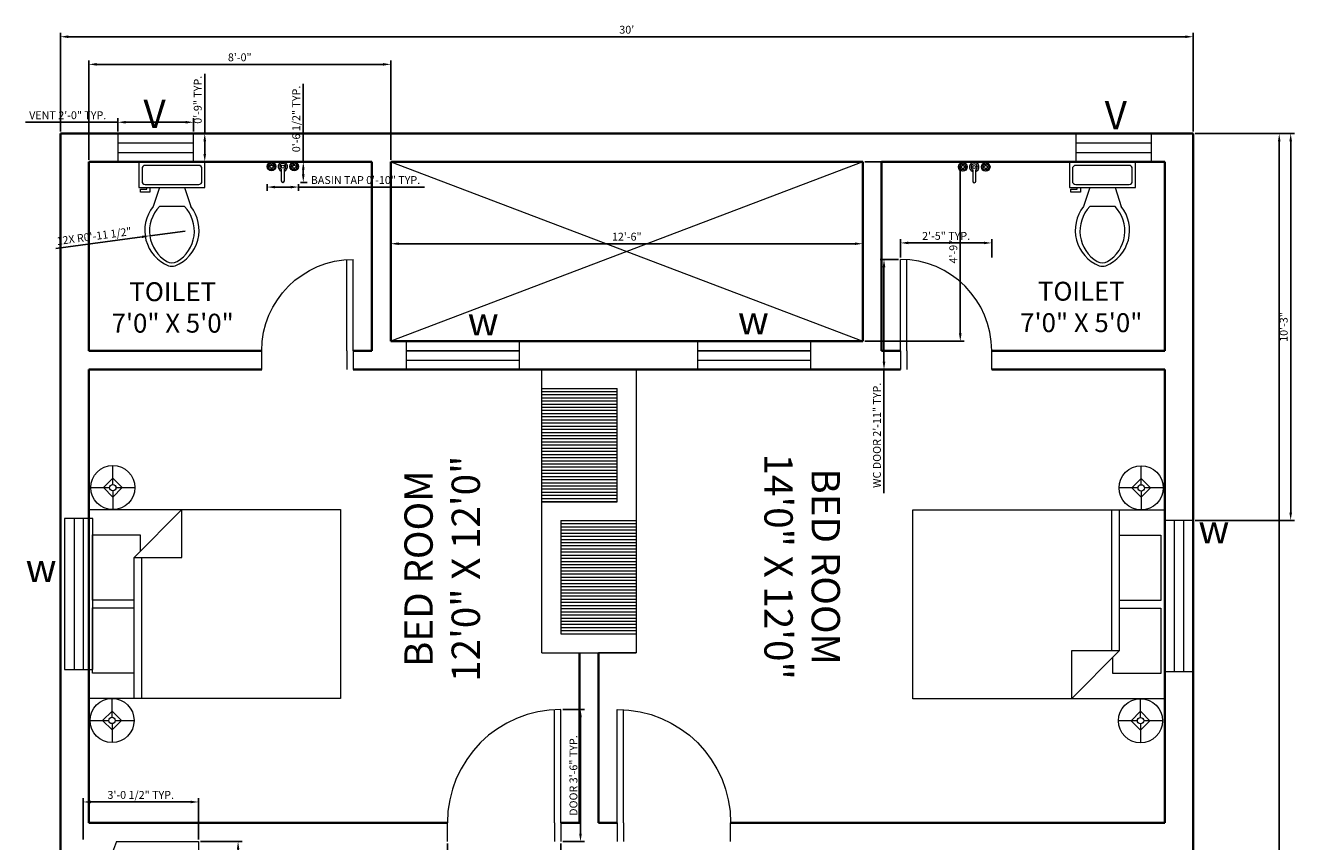
# Model space of a CAD drawing. Units: inches. Extents: x 2009 to 2890, y 2827 to 3504.
# Tile 6 of 6: x 2486 to 2890, y 3214 to 3473. Entities that reach past the tile are written whole.
import ezdxf

# ---------------------------------------------------------------- set-up
doc = ezdxf.new("R2010")
doc.units = ezdxf.units.IN
for name, color, linetype, lineweight in [('A-ANNO-DIMS', 2, 'Continuous', 18), ('A-ANNO-TEXT', 3, 'Continuous', 18), ('A-AREA-IDEN', 7, 'Continuous', 25), ('A-DOOR', 3, 'Continuous', 18), ('A-FLOR-CASE', 32, 'Continuous', 20), ('A-FLOR-FIXT', 9, 'Continuous', 18), ('A-FLOR-OPEN', 8, 'Continuous', 13), ('A-FLOR-PATT', 252, 'Continuous', 13), ('A-FURN', 8, 'Continuous', 18), ('A-GLAZ', 4, 'Continuous', 18), ('A-WALL', 7, 'Continuous', 35)]:
    doc.layers.add(name, color=color, linetype=linetype, lineweight=lineweight)
doc.styles.get("Standard").update_dxf_attribs({"font": 'arial.ttf'})
doc.dimstyles.new('ISO-25', dxfattribs={"dimtxt": 2.5, "dimasz": 2.5, "dimexe": 1.25, "dimexo": 0.625, "dimtad": 1, "dimdec": 0, "dimlunit": 3, "dimtxsty": 'Standard', "dimcen": 2.5, "dimadec": 0, "dimazin": 0, "dimtfac": 1, "dimtdec": 0, "dimtmove": 0, "dimatfit": 3, "dimfxl": 1, "dimarcsym": 0})

# ---------------------------------------------------------------- blocks, each defined once
blk = doc.blocks.new('*D13')
at = {"layer": 'A-ANNO-DIMS', "color": 0, "lineweight": -2, "transparency": 16777216}
for p, q in [((2497.61, 3439.57), (2497.61, 3470.97)), ((2500.11, 3469.72), (2855.11, 3469.72)), ((2857.61, 3439.57), (2857.61, 3470.97))]:
    blk.add_line(p, q, dxfattribs=at)
at = {"layer": 'A-ANNO-DIMS', "color": 0, "transparency": 16777216}
for points in [[(2500.11, 3470.14), (2500.11, 3469.3), (2497.61, 3469.72)], [(2855.11, 3470.14), (2855.11, 3469.3), (2857.61, 3469.72)]]:
    blk.add_solid(points, dxfattribs=at)
at = {"layer": 'Defpoints', "color": 0, "transparency": 16777216}
for p in [(2857.61, 3469.72), (2497.61, 3438.94), (2857.61, 3438.94)]:
    blk.add_point(p, dxfattribs=at)
at = {"layer": 'A-ANNO-DIMS', "color": 0, "transparency": 16777216, "insert": (2677.61, 3471.62), "char_height": 2.5, "attachment_point": 5}
blk.add_mtext("30'", dxfattribs=at)
blk = doc.blocks.new('*D14')
at = {"layer": 'A-ANNO-DIMS', "color": 0, "lineweight": -2, "transparency": 16777216}
for p, q in [((2858.24, 3438.94), (2886.22, 3438.94)), ((2884.97, 3436.44), (2884.97, 2901.44)), ((2870.41, 2898.94), (2886.22, 2898.94))]:
    blk.add_line(p, q, dxfattribs=at)
at = {"layer": 'A-ANNO-DIMS', "color": 0, "transparency": 16777216}
for points in [[(2884.55, 3436.44), (2885.39, 3436.44), (2884.97, 3438.94)], [(2884.55, 2901.44), (2885.39, 2901.44), (2884.97, 2898.94)]]:
    blk.add_solid(points, dxfattribs=at)
at = {"layer": 'Defpoints', "color": 0, "transparency": 16777216}
for p in [(2857.61, 3438.94), (2869.79, 2898.94), (2884.97, 2898.94)]:
    blk.add_point(p, dxfattribs=at)
at = {"layer": 'A-ANNO-DIMS', "color": 0, "transparency": 16777216, "insert": (2883.07, 3168.94), "char_height": 2.5, "attachment_point": 5, "rotation": 90}
blk.add_mtext("45'", dxfattribs=at)
blk = doc.blocks.new('Toilet - top')
for p, q in [((9.5, -6), (9.5, -2)), ((-8, -8.5), (-8, -8)), ((-7, -8), (-7, -9.5)), ((-4, -8), (-6, -14)), ((4, -8), (6, -14)), ((-10, -8.5), (-8, -8.5)), ((-10, -9.5), (-10, -8.5)), ((-7, -9.5), (-10, -9.5)), ((4, -14), (-4, -14))]:
    blk.add_line(p, q)
blk.add_lwpolyline([(10.5, -8), (10.5, 0), (-10.5, 0), (-10.5, -8)], close=True)
for points in [[(-9.5, -2), (-9.5, -6)], [(8.5, -1), (-8.5, -1)], [(-8.5, -7), (8.5, -7)]]:
    blk.add_lwpolyline(points)
for centre, radius, start, end in [((-8.62, -1.88), 0.884, 81.8699, 188.1301), ((8.62, -1.88), 0.884, 351.8699, 98.1301), ((-8.62, -6.12), 0.884, 171.8699, 278.1301), ((8.62, -6.12), 0.884, 261.8699, 8.1301), ((3.52, -21.58), 12.17, 141.4691, 247.9714), ((4.2, -21.82), 11.33, 136.3677, 238.9468), ((-3.52, -21.58), 12.17, 292.0284, 38.5307), ((-4.2, -21.82), 11.33, 301.053, 43.6321), ((0, -27.88), 4, 245.7318, 294.2682), ((0, -29), 4, 254.8605, 285.1395)]:
    blk.add_arc(centre, radius, start, end)
blk = doc.blocks.new('Sofa - Roundback 7 ft.')
for p, q in [((-12.00002, -32.4421), (-12.00003, -6.5971)), ((11.99997, -32.4421), (11.99998, -6.5971)), ((-36.000027, -34), (-36.000027, -11.4696)), ((35.99998, -34), (35.99998, -11.4696)), ((-35.999844, -13.3819), (35.9998, -13.3819)), ((-36.000027, -32.4421), (35.99998, -32.4421))]:
    blk.add_line(p, q)
for points in [[(-36.000027, -34), (-42.000027, -34), (-42.000027, -8)], [(41.99998, -8), (41.99998, -34), (35.99998, -34)]]:
    blk.add_lwpolyline(points)
for centre, radius, start, end in [((0, -114.25), 114.25, 68.43141, 111.5686), ((-0.00001, -127.1968), 121.1968, 72.72033, 107.2797)]:
    blk.add_arc(centre, radius, start, end)
blk = doc.blocks.new('Bed - Queen')
for p, q in [((0, -80.00003), (0, 0)), ((0, 0), (59.99999, 0)), ((59.99999, 0), (59.99999, -80.00003)), ((7.99999, -1.2), (28.79998, -1.2)), ((7.99999, -14.4), (7.99999, -1.2)), ((28.79998, -1.2), (28.79998, -14.4)), ((31.19999, -1.2), (51.99999, -1.2)), ((31.19999, -14.4), (31.19999, -1.2)), ((51.99999, -1.2), (51.99999, -16.4)), ((0, -14.4), (44.8, -14.4)), ((59.99999, -29.6), (44.8, -14.4)), ((44.8, -14.4), (44.8, -29.6)), ((44.8, -16.8), (0, -16.8)), ((51.99999, -16.4), (46.79936, -16.4)), ((44.8, -29.6), (59.99999, -29.6)), ((59.99999, -80.00003), (0, -80.00003))]:
    blk.add_line(p, q)
blk = doc.blocks.new('Lamp - Table')
for p, q in [((0, 7), (0, 1)), ((-1, 0), (-7, 0)), ((0, 3), (-3, 0)), ((-3, 0), (0, -3)), ((3, 0), (0, 3)), ((0, -3), (3, 0)), ((1, 0), (7, 0)), ((0, -1), (0, -7))]:
    blk.add_line(p, q)
for radius in [7, 1]:
    blk.add_circle((0, 0), radius)
blk = doc.blocks.new('Faucet - Bathroom top')
for p, q in [((-4.107, 0.125), (-4.375, 0.125)), ((-3.75, 0.4788), (-3.75, 0.75)), ((-3.5, 0.482), (-3.5, 0.75)), ((-3.1461, 0.125), (-2.875, 0.125)), ((3.143, 0.125), (2.875, 0.125)), ((3.5, 0.4788), (3.5, 0.75)), ((3.75, 0.482), (3.75, 0.75)), ((4.1039, 0.125), (4.375, 0.125)), ((-4.1039, -0.125), (-4.375, -0.125)), ((-3.75, -0.4821), (-3.75, -0.75)), ((-3.5, -0.4789), (-3.5, -0.75)), ((-3.143, -0.125), (-2.875, -0.125)), ((-0.5, -0.8639), (-0.5, -4.5)), ((0.5, -4.5), (0.5, -0.8631)), ((3.1461, -0.125), (2.875, -0.125)), ((3.5, -0.4821), (3.5, -0.75)), ((3.75, -0.4789), (3.75, -0.75)), ((4.107, -0.125), (4.375, -0.125))]:
    blk.add_line(p, q)
for centre, radius in [((-3.625, 0), 1.375), ((-4.625, 0), 0.2795), ((-3.625, 0), 0.5), ((-3.625, 1), 0.2795), ((-2.625, 0), 0.2795), ((0, 0), 0.5), ((3.625, 0), 1.375), ((2.625, 0), 0.2795), ((3.625, 0), 0.5), ((3.625, 1), 0.2795), ((4.625, 0), 0.2795), ((-3.625, -1), 0.2795), ((3.625, -1), 0.2795)]:
    blk.add_circle(centre, radius)
for centre, radius, start, end in [((-3.625, 0), 1, 105.2407, 164.2093), ((-3.625, 0), 1, 16.44125, 74.07887), ((0, 0), 1.5, 289.6514, 250.3603), ((0, 0), 1, 300.3431, 239.7554), ((3.625, 0), 1, 106.12, 164.0884), ((3.625, 0), 1, 16.23422, 73.90469), ((-3.625, 0), 1, 196.2342, 253.9047), ((-3.625, 0), 1, 286.12, 344.0884), ((3.625, 0), 1, 196.4413, 254.0789), ((3.625, 0), 1, 285.2407, 344.2093), ((0, -4.5), 0.5, 180, 0)]:
    blk.add_arc(centre, radius, start, end)
blk = doc.blocks.new('WIN-48IN')
for p, q in [((0, 48), (0, 0)), ((9, 48), (0, 48)), ((3, 48), (3, 0)), ((6, 0), (6, 48)), ((9, 0), (9, 48)), ((0, 0), (9, 0))]:
    blk.add_line(p, q)
blk = doc.blocks.new('WIN-36IN')
for p, q in [((0, 36), (0, 0)), ((9, 36), (0, 36)), ((3, 36), (3, 0)), ((6, 0), (6, 36)), ((9, 0), (9, 36)), ((0, 0), (9, 0))]:
    blk.add_line(p, q)
blk = doc.blocks.new('VENT-24IN')
for p, q in [((0, 24), (0, 0)), ((9, 24), (0, 24)), ((3, 24), (3, 0)), ((6, 0), (6, 24)), ((9, 0), (9, 24)), ((0, 0), (9, 0))]:
    blk.add_line(p, q)
blk = doc.blocks.new('DOOR-29IN')
for p, q in [((0, 35), (0, 29)), ((27, 29), (27, 35)), ((29, 29), (29, 35)), ((27, 29), (27, 0)), ((29, 29), (29, 0))]:
    blk.add_line(p, q)
blk.add_arc((29, 29), 29, 180, 270)
blk = doc.blocks.new('DOOR-36IN')
for p, q in [((34, 6), (34, 42)), ((36, 6), (36, 42)), ((0, 0), (0, 6)), ((34, 6), (34, 0)), ((36, 6), (36, 0))]:
    blk.add_line(p, q)
blk.add_arc((36, 6), 36, 90, 180)
blk = doc.blocks.new('*D35')
at = {"layer": 'A-ANNO-DIMS', "color": 0, "lineweight": -2, "transparency": 16777216}
for p, q in [((2515.89, 3442.54), (2486.48, 3442.54)), ((2515.89, 3439.57), (2515.89, 3443.79)), ((2537.39, 3442.54), (2518.39, 3442.54)), ((2539.89, 3439.57), (2539.89, 3443.79))]:
    blk.add_line(p, q, dxfattribs=at)
at = {"layer": 'A-ANNO-DIMS', "color": 0, "transparency": 16777216}
for points in [[(2518.39, 3442.96), (2518.39, 3442.13), (2515.89, 3442.54)], [(2537.39, 3442.96), (2537.39, 3442.13), (2539.89, 3442.54)]]:
    blk.add_solid(points, dxfattribs=at)
at = {"layer": 'Defpoints', "color": 0, "transparency": 16777216}
for p in [(2515.89, 3442.54), (2515.89, 3438.94), (2539.89, 3438.94)]:
    blk.add_point(p, dxfattribs=at)
at = {"layer": 'A-ANNO-DIMS', "color": 0, "transparency": 16777216, "insert": (2499.94, 3444.45), "char_height": 2.5, "attachment_point": 5}
blk.add_mtext('VENT 2\'-0" TYP.', dxfattribs=at)
blk = doc.blocks.new('*D36')
at = {"layer": 'A-ANNO-DIMS', "color": 0, "lineweight": -2, "transparency": 16777216}
for p, q in [((2543.49, 3438.94), (2543.49, 3457.93)), ((2540.51, 3438.94), (2544.74, 3438.94)), ((2543.49, 3432.44), (2543.49, 3436.44)), ((2540.51, 3429.94), (2544.74, 3429.94))]:
    blk.add_line(p, q, dxfattribs=at)
at = {"layer": 'A-ANNO-DIMS', "color": 0, "transparency": 16777216}
for points in [[(2543.07, 3436.44), (2543.9, 3436.44), (2543.49, 3438.94)], [(2543.07, 3432.44), (2543.9, 3432.44), (2543.49, 3429.94)]]:
    blk.add_solid(points, dxfattribs=at)
at = {"layer": 'Defpoints', "color": 0, "transparency": 16777216}
for p in [(2539.89, 3438.94), (2543.49, 3438.94), (2539.89, 3429.94)]:
    blk.add_point(p, dxfattribs=at)
at = {"layer": 'A-ANNO-DIMS', "color": 0, "transparency": 16777216, "insert": (2541.59, 3449.69), "char_height": 2.5, "attachment_point": 5, "rotation": 90}
blk.add_mtext('0\'-9" TYP.', dxfattribs=at)
blk = doc.blocks.new('*D37')
at = {"layer": 'A-ANNO-DIMS', "color": 0, "lineweight": -2, "transparency": 16777216}
for p, q in [((2657.24, 3255.94), (2664.16, 3255.94)), ((2662.91, 3216.44), (2662.91, 3253.44)), ((2657.24, 3213.94), (2664.16, 3213.94))]:
    blk.add_line(p, q, dxfattribs=at)
at = {"layer": 'A-ANNO-DIMS', "color": 0, "transparency": 16777216}
for points in [[(2662.49, 3253.44), (2663.33, 3253.44), (2662.91, 3255.94)], [(2662.49, 3216.44), (2663.33, 3216.44), (2662.91, 3213.94)]]:
    blk.add_solid(points, dxfattribs=at)
at = {"layer": 'Defpoints', "color": 0, "transparency": 16777216}
for p in [(2656.61, 3255.94), (2662.91, 3255.94), (2656.61, 3213.94)]:
    blk.add_point(p, dxfattribs=at)
at = {"layer": 'A-ANNO-DIMS', "color": 0, "transparency": 16777216, "insert": (2660.99, 3234.94), "char_height": 2.5, "attachment_point": 5, "rotation": 90}
blk.add_mtext('DOOR 3\'-6" TYP.', dxfattribs=at)
blk = doc.blocks.new('*D38')
at = {"layer": 'A-ANNO-DIMS', "color": 0, "lineweight": -2, "transparency": 16777216}
for p, q in [((2620.61, 3213.32), (2620.61, 3206.39)), ((2656.61, 3213.32), (2656.61, 3206.39)), ((2623.11, 3207.64), (2654.11, 3207.64))]:
    blk.add_line(p, q, dxfattribs=at)
at = {"layer": 'A-ANNO-DIMS', "color": 0, "transparency": 16777216}
for points in [[(2623.11, 3208.06), (2623.11, 3207.23), (2620.61, 3207.64)], [(2654.11, 3208.06), (2654.11, 3207.23), (2656.61, 3207.64)]]:
    blk.add_solid(points, dxfattribs=at)
at = {"layer": 'Defpoints', "color": 0, "transparency": 16777216}
for p in [(2620.61, 3213.94), (2656.61, 3213.94), (2656.61, 3207.64)]:
    blk.add_point(p, dxfattribs=at)
at = {"layer": 'A-ANNO-DIMS', "color": 0, "transparency": 16777216, "insert": (2638.61, 3209.55), "char_height": 2.5, "attachment_point": 5}
blk.add_mtext('3\'-0" TYP.', dxfattribs=at)
blk = doc.blocks.new('*D39')
at = {"layer": 'A-ANNO-DIMS', "color": 0, "lineweight": -2, "transparency": 16777216}
for p, q in [((2763.99, 3398.94), (2758.11, 3398.94)), ((2759.36, 3396.44), (2759.36, 3366.44)), ((2763.99, 3363.94), (2758.11, 3363.94)), ((2759.36, 3363.94), (2759.36, 3324.67))]:
    blk.add_line(p, q, dxfattribs=at)
at = {"layer": 'A-ANNO-DIMS', "color": 0, "transparency": 16777216}
for points in [[(2758.94, 3396.44), (2759.78, 3396.44), (2759.36, 3398.94)], [(2758.94, 3366.44), (2759.78, 3366.44), (2759.36, 3363.94)]]:
    blk.add_solid(points, dxfattribs=at)
at = {"layer": 'Defpoints', "color": 0, "transparency": 16777216}
for p in [(2764.61, 3398.94), (2759.36, 3363.94), (2764.61, 3363.94)]:
    blk.add_point(p, dxfattribs=at)
at = {"layer": 'A-ANNO-DIMS', "color": 0, "transparency": 16777216, "insert": (2757.44, 3343.06), "char_height": 2.5, "attachment_point": 5, "rotation": 90}
blk.add_mtext('WC DOOR 2\'-11" TYP.', dxfattribs=at)
blk = doc.blocks.new('*D40')
at = {"layer": 'A-ANNO-DIMS', "color": 0, "lineweight": -2, "transparency": 16777216}
for p, q in [((2764.61, 3399.57), (2764.61, 3405.44)), ((2793.61, 3399.57), (2793.61, 3405.44)), ((2791.11, 3404.19), (2767.11, 3404.19))]:
    blk.add_line(p, q, dxfattribs=at)
at = {"layer": 'A-ANNO-DIMS', "color": 0, "transparency": 16777216}
for points in [[(2767.11, 3404.61), (2767.11, 3403.78), (2764.61, 3404.19)], [(2791.11, 3404.61), (2791.11, 3403.78), (2793.61, 3404.19)]]:
    blk.add_solid(points, dxfattribs=at)
at = {"layer": 'Defpoints', "color": 0, "transparency": 16777216}
for p in [(2764.61, 3404.19), (2764.61, 3398.94), (2793.61, 3398.94)]:
    blk.add_point(p, dxfattribs=at)
at = {"layer": 'A-ANNO-DIMS', "color": 0, "transparency": 16777216, "insert": (2779.11, 3406.1), "char_height": 2.5, "attachment_point": 5}
blk.add_mtext('2\'-5" TYP.', dxfattribs=at)
blk = doc.blocks.new('*D49')
at = {"layer": 'A-ANNO-DIMS', "color": 0, "lineweight": -2, "transparency": 16777216}
for p, q in [((2563.31, 3422.82), (2563.31, 3420.7)), ((2565.81, 3421.95), (2570.81, 3421.95)), ((2573.31, 3422.82), (2573.31, 3420.7)), ((2573.31, 3421.95), (2613.34, 3421.95))]:
    blk.add_line(p, q, dxfattribs=at)
at = {"layer": 'A-ANNO-DIMS', "color": 0, "transparency": 16777216}
for points in [[(2565.81, 3422.36), (2565.81, 3421.53), (2563.31, 3421.95)], [(2570.81, 3422.36), (2570.81, 3421.53), (2573.31, 3421.95)]]:
    blk.add_solid(points, dxfattribs=at)
at = {"layer": 'Defpoints', "color": 0, "transparency": 16777216}
for p in [(2563.31, 3423.45), (2573.31, 3423.45), (2573.31, 3421.95)]:
    blk.add_point(p, dxfattribs=at)
at = {"layer": 'A-ANNO-DIMS', "color": 0, "transparency": 16777216, "insert": (2594.57, 3423.86), "char_height": 2.5, "attachment_point": 5}
blk.add_mtext('BASIN TAP 0\'-10" TYP.', dxfattribs=at)
blk = doc.blocks.new('*D50')
at = {"layer": 'A-ANNO-DIMS', "color": 0, "lineweight": -2, "transparency": 16777216}
for p, q in [((2574.81, 3429.95), (2574.81, 3454.76)), ((2573.93, 3429.95), (2576.06, 3429.95)), ((2574.81, 3425.95), (2574.81, 3427.45)), ((2573.93, 3423.45), (2576.06, 3423.45))]:
    blk.add_line(p, q, dxfattribs=at)
at = {"layer": 'A-ANNO-DIMS', "color": 0, "transparency": 16777216}
for points in [[(2574.39, 3427.45), (2575.22, 3427.45), (2574.81, 3429.95)], [(2574.39, 3425.95), (2575.22, 3425.95), (2574.81, 3423.45)]]:
    blk.add_solid(points, dxfattribs=at)
at = {"layer": 'Defpoints', "color": 0, "transparency": 16777216}
for p in [(2573.31, 3429.95), (2574.81, 3429.95), (2573.31, 3423.45)]:
    blk.add_point(p, dxfattribs=at)
at = {"layer": 'A-ANNO-DIMS', "color": 0, "transparency": 16777216, "insert": (2572.89, 3443.6), "char_height": 2.5, "attachment_point": 5, "rotation": 90}
blk.add_mtext('0\'-6 1/2" TYP.', dxfattribs=at)
blk = doc.blocks.new('*D51')
at = {"layer": 'A-ANNO-DIMS', "color": 0, "lineweight": -2, "transparency": 16777216}
for p, q in [((2542.11, 3213.94), (2555.33, 3213.94)), ((2554.08, 3132.44), (2554.08, 3211.44)), ((2542.11, 3129.94), (2555.33, 3129.94))]:
    blk.add_line(p, q, dxfattribs=at)
at = {"layer": 'A-ANNO-DIMS', "color": 0, "transparency": 16777216}
for points in [[(2553.67, 3211.44), (2554.5, 3211.44), (2554.08, 3213.94)], [(2553.67, 3132.44), (2554.5, 3132.44), (2554.08, 3129.94)]]:
    blk.add_solid(points, dxfattribs=at)
at = {"layer": 'Defpoints', "color": 0, "transparency": 16777216}
for p in [(2541.48, 3213.94), (2554.08, 3213.94), (2541.48, 3129.94)]:
    blk.add_point(p, dxfattribs=at)
at = {"layer": 'A-ANNO-DIMS', "color": 0, "transparency": 16777216, "insert": (2552.16, 3171.94), "char_height": 2.5, "attachment_point": 5, "rotation": 90}
blk.add_mtext('SOFA 7\'-0" TYP.', dxfattribs=at)
blk = doc.blocks.new('*D52')
at = {"layer": 'A-ANNO-DIMS', "color": 0, "lineweight": -2, "transparency": 16777216}
for p, q in [((2504.82, 3214.57), (2504.82, 3227.79)), ((2541.48, 3214.57), (2541.48, 3227.79)), ((2538.98, 3226.54), (2507.32, 3226.54))]:
    blk.add_line(p, q, dxfattribs=at)
at = {"layer": 'A-ANNO-DIMS', "color": 0, "transparency": 16777216}
for points in [[(2507.32, 3226.96), (2507.32, 3226.13), (2504.82, 3226.54)], [(2538.98, 3226.96), (2538.98, 3226.13), (2541.48, 3226.54)]]:
    blk.add_solid(points, dxfattribs=at)
at = {"layer": 'Defpoints', "color": 0, "transparency": 16777216}
for p in [(2504.82, 3226.54), (2504.82, 3213.94), (2541.48, 3213.94)]:
    blk.add_point(p, dxfattribs=at)
at = {"layer": 'A-ANNO-DIMS', "color": 0, "transparency": 16777216, "insert": (2523.15, 3228.46), "char_height": 2.5, "attachment_point": 5}
blk.add_mtext('3\'-0 1/2" TYP.', dxfattribs=at)
blk = doc.blocks.new('*D70')
at = {"layer": 'A-ANNO-DIMS', "color": 0, "lineweight": -2, "transparency": 16777216}
for p, q in [((2602.61, 3373.57), (2602.61, 3405.19)), ((2752.61, 3373.57), (2752.61, 3405.19)), ((2605.11, 3403.94), (2750.11, 3403.94))]:
    blk.add_line(p, q, dxfattribs=at)
at = {"layer": 'A-ANNO-DIMS', "color": 0, "transparency": 16777216}
for points in [[(2605.11, 3404.36), (2605.11, 3403.53), (2602.61, 3403.94)], [(2750.11, 3404.36), (2750.11, 3403.53), (2752.61, 3403.94)]]:
    blk.add_solid(points, dxfattribs=at)
at = {"layer": 'Defpoints', "color": 0, "transparency": 16777216}
for p in [(2752.61, 3403.94), (2602.61, 3372.94), (2752.61, 3372.94)]:
    blk.add_point(p, dxfattribs=at)
at = {"layer": 'A-ANNO-DIMS', "color": 0, "transparency": 16777216, "insert": (2677.61, 3405.85), "char_height": 2.5, "attachment_point": 5}
blk.add_mtext('12\'-6"', dxfattribs=at)
blk = doc.blocks.new('*D71')
at = {"layer": 'A-ANNO-DIMS', "color": 0, "lineweight": -2, "transparency": 16777216}
for p, q in [((2753.24, 3429.94), (2784.86, 3429.94)), ((2783.61, 3427.44), (2783.61, 3375.44)), ((2753.24, 3372.94), (2784.86, 3372.94))]:
    blk.add_line(p, q, dxfattribs=at)
at = {"layer": 'A-ANNO-DIMS', "color": 0, "transparency": 16777216}
for points in [[(2783.19, 3427.44), (2784.03, 3427.44), (2783.61, 3429.94)], [(2783.19, 3375.44), (2784.03, 3375.44), (2783.61, 3372.94)]]:
    blk.add_solid(points, dxfattribs=at)
at = {"layer": 'Defpoints', "color": 0, "transparency": 16777216}
for p in [(2752.61, 3429.94), (2752.61, 3372.94), (2783.61, 3372.94)]:
    blk.add_point(p, dxfattribs=at)
at = {"layer": 'A-ANNO-DIMS', "color": 0, "transparency": 16777216, "insert": (2781.71, 3401.44), "char_height": 2.5, "attachment_point": 5, "rotation": 90}
blk.add_mtext('4\'-9"', dxfattribs=at)
blk = doc.blocks.new('*D78')
at = {"layer": 'A-ANNO-DIMS', "color": 0, "lineweight": -2, "transparency": 16777216}
for p, q in [((2506.61, 3430.57), (2506.61, 3462.19)), ((2602.61, 3430.57), (2602.61, 3462.19)), ((2509.11, 3460.94), (2600.11, 3460.94))]:
    blk.add_line(p, q, dxfattribs=at)
at = {"layer": 'A-ANNO-DIMS', "color": 0, "transparency": 16777216}
for points in [[(2509.11, 3461.36), (2509.11, 3460.53), (2506.61, 3460.94)], [(2600.11, 3461.36), (2600.11, 3460.53), (2602.61, 3460.94)]]:
    blk.add_solid(points, dxfattribs=at)
at = {"layer": 'Defpoints', "color": 0, "transparency": 16777216}
for p in [(2602.61, 3460.94), (2506.61, 3429.94), (2602.61, 3429.94)]:
    blk.add_point(p, dxfattribs=at)
at = {"layer": 'A-ANNO-DIMS', "color": 0, "transparency": 16777216, "insert": (2554.61, 3462.85), "char_height": 2.5, "attachment_point": 5}
blk.add_mtext('8\'-0"', dxfattribs=at)
blk = doc.blocks.new('*D82')
at = {"layer": 'A-ANNO-DIMS', "color": 0, "lineweight": -2, "transparency": 16777216}
for p, q in [((2858.24, 3438.94), (2889.86, 3438.94)), ((2888.61, 3436.44), (2888.61, 3318.53)), ((2858.24, 3316.03), (2889.86, 3316.03))]:
    blk.add_line(p, q, dxfattribs=at)
at = {"layer": 'A-ANNO-DIMS', "color": 0, "transparency": 16777216}
for points in [[(2888.19, 3436.44), (2889.03, 3436.44), (2888.61, 3438.94)], [(2888.19, 3318.53), (2889.03, 3318.53), (2888.61, 3316.03)]]:
    blk.add_solid(points, dxfattribs=at)
at = {"layer": 'Defpoints', "color": 0, "transparency": 16777216}
for p in [(2857.61, 3438.94), (2857.61, 3316.03), (2888.61, 3316.03)]:
    blk.add_point(p, dxfattribs=at)
at = {"layer": 'A-ANNO-DIMS', "color": 0, "transparency": 16777216, "insert": (2886.71, 3377.49), "char_height": 2.5, "attachment_point": 5, "rotation": 90}
blk.add_mtext('10\'-3"', dxfattribs=at)
blk = doc.blocks.new('*D92')
at = {"layer": 'A-ANNO-DIMS', "color": 0, "lineweight": -2, "transparency": 16777216}
for p, q in [((2496.16, 3402.45), (2523.55, 3406.13)), ((2537.26, 3407.97), (2526.03, 3406.47))]:
    blk.add_line(p, q, dxfattribs=at)
at = {"layer": 'A-ANNO-DIMS', "color": 0, "transparency": 16777216}
blk.add_solid([(2523.49, 3406.54), (2523.6, 3405.72), (2526.03, 3406.47)], dxfattribs=at)
at = {"layer": 'Defpoints', "color": 0, "transparency": 16777216}
for p in [(2526.03, 3406.47), (2537.26, 3407.97)]:
    blk.add_point(p, dxfattribs=at)
at = {"layer": 'A-ANNO-DIMS', "color": 0, "transparency": 16777216, "insert": (2508.36, 3406.02), "char_height": 2.5, "attachment_point": 5, "rotation": 7.6592}
blk.add_mtext('12X R0\'-11 1/2"', dxfattribs=at)

msp = doc.modelspace()

# ---------------------------------------------------------------- hatches: boundary and pattern name
at = {"layer": 'A-FLOR-PATT'}
h = msp.add_hatch(dxfattribs=at)
h.set_pattern_fill('ANSI31', color=256, scale=0.3149606, angle=-45, style=0)
h.paths.add_polyline_path([(2650.61, 3321.94), (2674.61, 3321.94), (2674.61, 3357.94), (2650.61, 3357.94)])
h = msp.add_hatch(dxfattribs=at)
h.set_pattern_fill('ANSI31', color=256, scale=0.3149606, angle=-45, style=0)
h.paths.add_polyline_path([(2656.61, 3279.94), (2680.61, 3279.94), (2680.61, 3315.94), (2656.61, 3315.94)])

# ---------------------------------------------------------------- linework, layer by layer
at = {"layer": 'A-FLOR-CASE'}
for p, q in [((2650.61, 3273.94), (2650.61, 3363.94)), ((2680.61, 3363.94), (2680.61, 3273.94)), ((2650.61, 3357.94), (2674.61, 3357.94)), ((2674.61, 3321.94), (2674.61, 3357.94)), ((2650.61, 3321.94), (2674.61, 3321.94)), ((2656.61, 3315.94), (2680.61, 3315.94)), ((2656.61, 3315.94), (2656.61, 3279.94)), ((2656.61, 3279.94), (2680.61, 3279.94)), ((2650.61, 3273.94), (2680.61, 3273.94)), ((2650.61, 3273.94), (2662.61, 3273.94)), ((2680.61, 3273.94), (2668.61, 3273.94))]:
    msp.add_line(p, q, dxfattribs=at)
at = {"layer": 'A-FLOR-OPEN'}
for p, q in [((2602.61, 3429.94), (2752.61, 3372.94)), ((2752.61, 3429.94), (2602.61, 3372.94))]:
    msp.add_line(p, q, dxfattribs=at)
at = {"layer": 'A-GLAZ'}
for p, q in [((2607.51, 3369.94), (2643.51, 3369.94)), ((2700.1, 3369.94), (2736.1, 3369.94))]:
    msp.add_line(p, q, dxfattribs=at)
at = {"layer": 'A-WALL'}
for p, q in [((2497.61, 3438.94), (2857.61, 3438.94)), ((2497.61, 2898.94), (2497.61, 3438.94)), ((2857.61, 3438.94), (2857.61, 2898.94)), ((2506.61, 3429.94), (2596.61, 3429.94)), ((2506.61, 3369.94), (2506.61, 3429.94)), ((2596.61, 3369.94), (2596.61, 3429.94)), ((2602.61, 3372.94), (2602.61, 3429.94)), ((2602.61, 3429.94), (2752.61, 3429.94)), ((2752.61, 3429.94), (2752.61, 3372.94)), ((2752.61, 3372.94), (2752.61, 3429.94)), ((2752.61, 3372.94), (2752.61, 3429.94)), ((2758.61, 3429.94), (2758.61, 3369.94)), ((2758.61, 3429.94), (2848.61, 3429.94)), ((2848.61, 3429.94), (2848.61, 3369.94)), ((2602.61, 3372.94), (2752.61, 3372.94)), ((2506.61, 3369.94), (2561.61, 3369.94)), ((2596.61, 3369.94), (2590.61, 3369.94)), ((2590.61, 3369.94), (2596.61, 3369.94)), ((2758.61, 3369.94), (2764.61, 3369.94)), ((2758.61, 3369.94), (2764.61, 3369.94)), ((2793.61, 3369.94), (2848.61, 3369.94)), ((2506.61, 3363.94), (2561.61, 3363.94)), ((2506.61, 3219.94), (2506.61, 3363.94)), ((2590.61, 3363.94), (2764.61, 3363.94)), ((2793.61, 3363.94), (2848.61, 3363.94)), ((2848.61, 3363.94), (2848.61, 3219.94)), ((2662.61, 3273.94), (2662.61, 3219.94)), ((2668.61, 3273.94), (2668.61, 3219.94)), ((2506.61, 3219.94), (2620.61, 3219.94)), ((2662.61, 3219.94), (2656.61, 3219.94)), ((2656.61, 3219.94), (2662.61, 3219.94)), ((2668.61, 3219.94), (2674.61, 3219.94)), ((2668.61, 3219.94), (2674.61, 3219.94)), ((2710.61, 3219.94), (2848.61, 3219.94))]:
    msp.add_line(p, q, dxfattribs=at)

# ---------------------------------------------------------------- block references
at = {"layer": 'A-DOOR', "extrusion": (0, 0, -1), "zscale": -1, "rotation": 180}
msp.add_blockref('DOOR-29IN', (-2561.61, 3398.94), dxfattribs=at)
at = {"layer": 'A-DOOR', "rotation": 180}
msp.add_blockref('DOOR-29IN', (2793.61, 3398.94), dxfattribs=at)
at = {"layer": 'A-DOOR'}
msp.add_blockref('DOOR-36IN', (2620.61, 3213.94), dxfattribs=at)
at = {"layer": 'A-DOOR', "extrusion": (0, 0, -1), "zscale": -1}
msp.add_blockref('DOOR-36IN', (-2710.61, 3213.94), dxfattribs=at)
at = {"layer": 'A-FLOR-FIXT'}
for name, p in [('Toilet - top', (2533.06, 3429.79)), ('Faucet - Bathroom top', (2568.31, 3428.45)), ('Faucet - Bathroom top', (2788.05, 3428.33)), ('Toilet - top', (2828.78, 3429.79))]:
    msp.add_blockref(name, p, dxfattribs=at)
at = {"layer": 'A-FURN'}
for name, p, rotation in [('Lamp - Table', (2514.26, 3326.45), 89.99999999999999), ('Lamp - Table', (2841.11, 3326.35), 270), ('Bed - Queen', (2506.61, 3259.45), 89.99999999999999), ('Bed - Queen', (2848.53, 3319.35), 270), ('Lamp - Table', (2514.03, 3252.45), 89.99999999999999), ('Lamp - Table', (2840.89, 3252.35), 270), ('Sofa - Roundback 7 ft.', (2507.48, 3171.94), 90)]:
    msp.add_blockref(name, p, dxfattribs=dict(at, rotation=rotation))
at = {"layer": 'A-GLAZ'}
for name, p, rotation in [('VENT-24IN', (2539.89, 3429.94), 90.00000000000193), ('VENT-24IN', (2844.37, 3429.94), 90.00000000000193), ('WIN-36IN', (2643.51, 3363.94), 89.99999999999966), ('WIN-36IN', (2736.1, 3363.94), 90.00000000000134)]:
    msp.add_blockref(name, p, dxfattribs=dict(at, rotation=rotation))
for p in [(2498.95, 3268.66), (2848.61, 3268.03)]:
    msp.add_blockref('WIN-48IN', p, dxfattribs=at)

# ---------------------------------------------------------------- texts
at = {"layer": 'A-ANNO-TEXT', "char_height": 9, "attachment_point": 1}
for s, width, insert in [('\\pxqc;V', 57.7621, (2498.66, 3449.69)), ('\\pxqc;V', 57.7621, (2804.14, 3449.3)), ('\\pxqc;w', 53.6341, (2605.16, 3383.81)), ('\\pxqc;w', 53.6341, (2691.03, 3384.18)), ('\\pxqc;w', 53.6341, (2837.38, 3317.75)), ('\\pxqc;w', 53.6341, (2464.66, 3305.48))]:
    msp.add_mtext_dynamic_manual_height_columns(s, width=width, gutter_width=12.5, heights=[0], dxfattribs=dict(at, insert=insert))
at = {"layer": 'A-AREA-IDEN', "char_height": 6, "attachment_point": 1}
for insert in [(2506.61, 3391.69), (2795.37, 3391.85)]:
    msp.add_mtext_dynamic_manual_height_columns('\\pxqc;TOILET\\P7\'0" X 5\'0"', width=53.3807, gutter_width=12.5, heights=[0], dxfattribs=dict(at, insert=insert))
at = {"layer": 'A-AREA-IDEN', "char_height": 9, "attachment_point": 1}
for s, insert, rotation in [('\\pxqc;BED ROOM\\P14\'0" X 12\'0" ', (2745.36, 3343.99), 270), ('\\pxqc;BED ROOM\\P12\'0" X 12\'0" ', (2606.94, 3257.99), 90)]:
    msp.add_mtext_dynamic_manual_height_columns(s, width=85.3364, gutter_width=12.5, heights=[0], dxfattribs=dict(at, insert=insert, rotation=rotation))

# ---------------------------------------------------------------- dimensions: what is measured, and where the dimension line sits
at = {"layer": 'A-ANNO-DIMS'}
for base, p1, p2, override, picture, middle in [((2857.61, 3469.72), (2497.61, 3438.94), (2857.61, 3438.94), {"dimclrd": 0, "dimclre": 0, "dimclrt": 0}, '*D13', (2677.61, 3471.62)), ((2602.61, 3460.94), (2506.61, 3429.94), (2602.61, 3429.94), {"dimdec": 1, "dimlfac": 1, "dimrnd": 0, "dimzin": 1, "dimdsep": 46, "dimlunit": 4, "dimfrac": 2}, '*D78', (2554.61, 3462.85))]:
    dim = msp.add_linear_dim(base=base, p1=p1, p2=p2, dimstyle='ISO-25', override=override, dxfattribs=at)
    dim.commit()
    dim.dimension.update_dxf_attribs({"geometry": picture, "text_midpoint": middle})
for base, p1, p2, angle, text, picture, middle in [((2543.49, 3438.94), (2539.89, 3429.94), (2539.89, 3438.94), 90, '<> TYP.', '*D36', (2541.59, 3449.69)), ((2574.81, 3429.95), (2573.31, 3423.45), (2573.31, 3429.95), 90, '<> TYP.', '*D50', (2572.89, 3443.6)), ((2515.89, 3442.54), (2539.89, 3438.94), (2515.89, 3438.94), 180, 'VENT <> TYP.', '*D35', (2499.94, 3444.45)), ((2764.61, 3404.19), (2793.61, 3398.94), (2764.61, 3398.94), 180, '<> TYP.', '*D40', (2779.11, 3406.1)), ((2759.36, 3363.94), (2764.61, 3398.94), (2764.61, 3363.94), 270, 'WC DOOR <> TYP.', '*D39', (2757.44, 3343.06)), ((2662.91, 3255.94), (2656.61, 3213.94), (2656.61, 3255.94), 90, 'DOOR <> TYP.', '*D37', (2660.99, 3234.94)), ((2504.82, 3226.54), (2541.48, 3213.94), (2504.82, 3213.94), 180, '<> TYP.', '*D52', (2523.15, 3228.46)), ((2554.08, 3213.94), (2541.48, 3129.94), (2541.48, 3213.94), 90, 'SOFA <> TYP.', '*D51', (2552.16, 3171.94))]:
    dim = msp.add_linear_dim(base=base, p1=p1, p2=p2, angle=angle, text=text, dimstyle='ISO-25', override={"dimdec": 1, "dimlfac": 1, "dimrnd": 0, "dimzin": 1, "dimdsep": 46, "dimlunit": 4, "dimfrac": 2}, dxfattribs=at)
    dim.commit()
    dim.dimension.update_dxf_attribs({"geometry": picture, "text_midpoint": middle})
for base, p1, p2, angle, override, picture, middle in [((2884.97, 2898.94), (2857.61, 3438.94), (2869.79, 2898.94), 90, {"dimclrd": 0, "dimclre": 0, "dimclrt": 0}, '*D14', (2883.07, 3168.94)), ((2888.61, 3316.03), (2857.61, 3438.94), (2857.61, 3316.03), 90, {"dimdec": 1, "dimlfac": 1, "dimrnd": 0, "dimzin": 1, "dimdsep": 46, "dimlunit": 4, "dimfrac": 2}, '*D82', (2886.71, 3377.49)), ((2783.61, 3372.94), (2752.61, 3429.94), (2752.61, 3372.94), 270, {"dimdec": 1, "dimlfac": 1, "dimrnd": 0, "dimzin": 1, "dimdsep": 46, "dimlunit": 4, "dimfrac": 2}, '*D71', (2781.71, 3401.44)), ((2752.61, 3403.94), (2602.61, 3372.94), (2752.61, 3372.94), 0, {"dimdec": 1, "dimlfac": 1, "dimrnd": 0, "dimzin": 1, "dimdsep": 46, "dimlunit": 4, "dimfrac": 2}, '*D70', (2677.61, 3405.85))]:
    dim = msp.add_linear_dim(base=base, p1=p1, p2=p2, angle=angle, dimstyle='ISO-25', override=override, dxfattribs=at)
    dim.commit()
    dim.dimension.update_dxf_attribs({"geometry": picture, "text_midpoint": middle})
for base, p1, p2, text, picture, middle in [((2573.31, 3421.95), (2563.31, 3423.45), (2573.31, 3423.45), 'BASIN TAP <> TYP.', '*D49', (2594.57, 3423.86)), ((2656.61, 3207.64), (2620.61, 3213.94), (2656.61, 3213.94), '<> TYP.', '*D38', (2638.61, 3209.55))]:
    dim = msp.add_linear_dim(base=base, p1=p1, p2=p2, text=text, dimstyle='ISO-25', override={"dimdec": 1, "dimlfac": 1, "dimrnd": 0, "dimzin": 1, "dimdsep": 46, "dimlunit": 4, "dimfrac": 2}, dxfattribs=at)
    dim.commit()
    dim.dimension.update_dxf_attribs({"geometry": picture, "text_midpoint": middle})
dim = msp.add_radius_dim(center=(2537.26, 3407.97), mpoint=(2526.03, 3406.47), text='12X <>', dimstyle='ISO-25', override={"dimdec": 1, "dimlfac": 1, "dimrnd": 0, "dimzin": 1, "dimdsep": 46, "dimlunit": 4, "dimfrac": 2}, dxfattribs=at)
dim.commit()
dim.dimension.update_dxf_attribs({"geometry": '*D92', "text_midpoint": (2508.36, 3406.02)})

doc.saveas('drawing.dxf')
